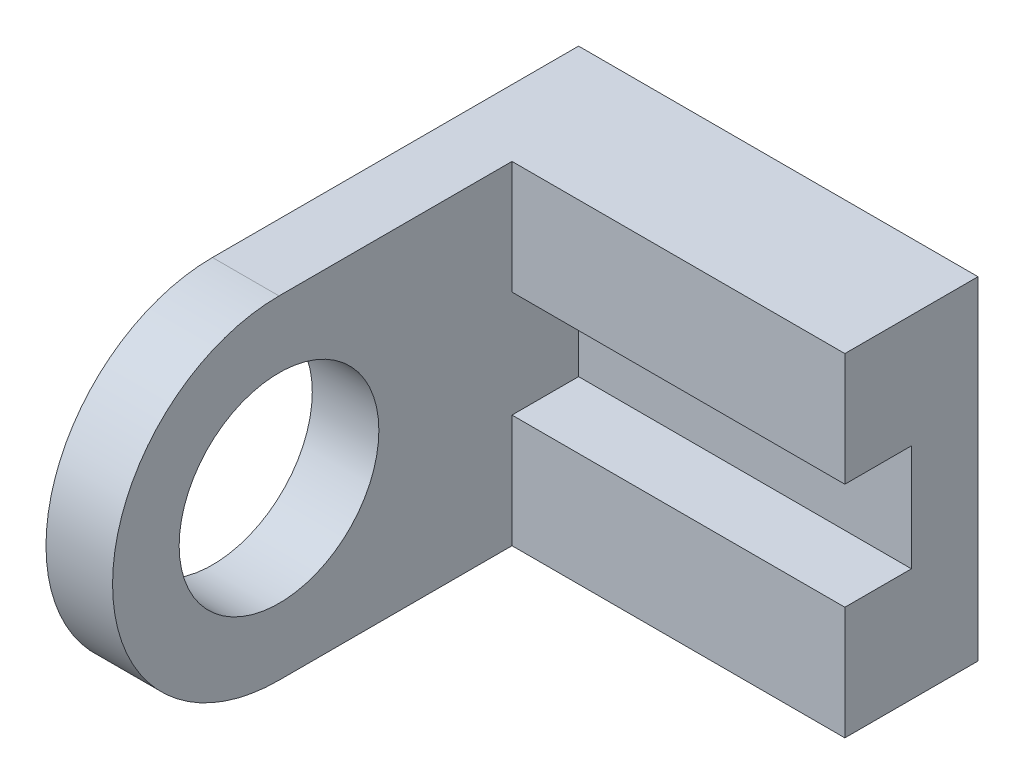
ISO-10303-21;
HEADER;
FILE_DESCRIPTION(('STEP AP214'),'2;1');
FILE_NAME('part.step','',(''),(''),'','','');
FILE_SCHEMA(('AUTOMOTIVE_DESIGN { 1 0 10303 214 1 1 1 1 }'));
ENDSEC;
DATA;
#1=APPLICATION_CONTEXT('core data for automotive mechanical design processes');
#2=APPLICATION_PROTOCOL_DEFINITION('international standard','automotive_design',2000,#1);
#3=PRODUCT_CONTEXT('',#1,'mechanical');
#4=PRODUCT('Part','Part','',(#3));
#5=PRODUCT_RELATED_PRODUCT_CATEGORY('part','',(#4));
#6=PRODUCT_DEFINITION_FORMATION('','',#4);
#7=PRODUCT_DEFINITION_CONTEXT('part definition',#1,'design');
#8=PRODUCT_DEFINITION('design','',#6,#7);
#9=PRODUCT_DEFINITION_SHAPE('','',#8);
#10=(LENGTH_UNIT() NAMED_UNIT(*) SI_UNIT(.MILLI.,.METRE.));
#11=(NAMED_UNIT(*) PLANE_ANGLE_UNIT() SI_UNIT($,.RADIAN.));
#12=(NAMED_UNIT(*) SI_UNIT($,.STERADIAN.) SOLID_ANGLE_UNIT());
#13=UNCERTAINTY_MEASURE_WITH_UNIT(LENGTH_MEASURE(1.E-05),#10,'distance_accuracy_value','');
#14=(GEOMETRIC_REPRESENTATION_CONTEXT(3) GLOBAL_UNCERTAINTY_ASSIGNED_CONTEXT((#13)) GLOBAL_UNIT_ASSIGNED_CONTEXT((#10,
#11,#12)) REPRESENTATION_CONTEXT('',''));
#15=CARTESIAN_POINT('',(0.,0.,0.));
#16=DIRECTION('',(0.,0.,1.));
#17=DIRECTION('',(1.,0.,0.));
#18=AXIS2_PLACEMENT_3D('',#15,#16,#17);
#19=CARTESIAN_POINT('',(0.,0.,10.));
#20=DIRECTION('',(0.,0.,1.));
#21=DIRECTION('',(1.,0.,0.));
#22=AXIS2_PLACEMENT_3D('',#19,#20,#21);
#23=PLANE('',#22);
#24=DIRECTION('',(1.,0.,0.));
#25=VECTOR('',#24,1.);
#26=CARTESIAN_POINT('',(0.,33.,10.));
#27=LINE('',#26,#25);
#28=CARTESIAN_POINT('',(10.,33.,10.));
#29=VERTEX_POINT('',#28);
#30=CARTESIAN_POINT('',(60.,33.,10.));
#31=VERTEX_POINT('',#30);
#32=EDGE_CURVE('E178',#29,#31,#27,.T.);
#33=ORIENTED_EDGE('',*,*,#32,.F.);
#34=DIRECTION('',(0.,-1.,0.));
#35=VECTOR('',#34,1.);
#36=CARTESIAN_POINT('',(10.,50.,10.));
#37=LINE('',#36,#35);
#38=CARTESIAN_POINT('',(10.,17.,10.));
#39=VERTEX_POINT('',#38);
#40=EDGE_CURVE('E131',#29,#39,#37,.T.);
#41=ORIENTED_EDGE('',*,*,#40,.T.);
#42=DIRECTION('',(1.,0.,0.));
#43=VECTOR('',#42,1.);
#44=CARTESIAN_POINT('',(0.,17.,10.));
#45=LINE('',#44,#43);
#46=CARTESIAN_POINT('',(60.,17.,10.));
#47=VERTEX_POINT('',#46);
#48=EDGE_CURVE('E167',#39,#47,#45,.T.);
#49=ORIENTED_EDGE('',*,*,#48,.T.);
#50=DIRECTION('',(0.,1.,0.));
#51=VECTOR('',#50,1.);
#52=CARTESIAN_POINT('',(60.,0.,10.));
#53=LINE('',#52,#51);
#54=EDGE_CURVE('E184',#47,#31,#53,.T.);
#55=ORIENTED_EDGE('',*,*,#54,.T.);
#56=EDGE_LOOP('',(#33,#41,#49,#55));
#57=FACE_BOUND('',#56,.T.);
#58=ADVANCED_FACE('F44',(#57),#23,.T.);
#59=CARTESIAN_POINT('',(0.,50.,10.));
#60=DIRECTION('',(1.,0.,0.));
#61=DIRECTION('',(0.,0.,-1.));
#62=AXIS2_PLACEMENT_3D('',#59,#60,#61);
#63=PLANE('',#62);
#64=CARTESIAN_POINT('',(0.,25.,55.));
#65=DIRECTION('',(1.,0.,0.));
#66=DIRECTION('',(0.,0.,-1.));
#67=AXIS2_PLACEMENT_3D('',#64,#65,#66);
#68=CIRCLE('',#67,15.);
#69=CARTESIAN_POINT('',(0.,25.,40.));
#70=VERTEX_POINT('',#69);
#71=EDGE_CURVE('E153',#70,#70,#68,.T.);
#72=ORIENTED_EDGE('',*,*,#71,.T.);
#73=EDGE_LOOP('',(#72));
#74=FACE_BOUND('',#73,.T.);
#75=DIRECTION('',(0.,0.,-1.));
#76=VECTOR('',#75,1.);
#77=CARTESIAN_POINT('',(0.,0.,10.));
#78=LINE('',#77,#76);
#79=CARTESIAN_POINT('',(0.,0.,55.));
#80=VERTEX_POINT('',#79);
#81=CARTESIAN_POINT('',(0.,0.,0.));
#82=VERTEX_POINT('',#81);
#83=EDGE_CURVE('E52',#80,#82,#78,.T.);
#84=ORIENTED_EDGE('',*,*,#83,.F.);
#85=CARTESIAN_POINT('',(0.,25.,55.));
#86=DIRECTION('',(-1.,0.,0.));
#87=DIRECTION('',(0.,0.,1.));
#88=AXIS2_PLACEMENT_3D('',#85,#86,#87);
#89=CIRCLE('',#88,25.);
#90=CARTESIAN_POINT('',(0.,50.,55.));
#91=VERTEX_POINT('',#90);
#92=EDGE_CURVE('E143',#80,#91,#89,.T.);
#93=ORIENTED_EDGE('',*,*,#92,.T.);
#94=DIRECTION('',(0.,0.,-1.));
#95=VECTOR('',#94,1.);
#96=CARTESIAN_POINT('',(0.,50.,10.));
#97=LINE('',#96,#95);
#98=CARTESIAN_POINT('',(0.,50.,0.));
#99=VERTEX_POINT('',#98);
#100=EDGE_CURVE('E58',#91,#99,#97,.T.);
#101=ORIENTED_EDGE('',*,*,#100,.T.);
#102=DIRECTION('',(0.,-1.,0.));
#103=VECTOR('',#102,1.);
#104=CARTESIAN_POINT('',(0.,50.,0.));
#105=LINE('',#104,#103);
#106=EDGE_CURVE('E179',#99,#82,#105,.T.);
#107=ORIENTED_EDGE('',*,*,#106,.T.);
#108=EDGE_LOOP('',(#84,#93,#101,#107));
#109=FACE_BOUND('',#108,.T.);
#110=ADVANCED_FACE('F50',(#74,#109),#63,.F.);
#111=CARTESIAN_POINT('',(0.,0.,10.));
#112=DIRECTION('',(0.,1.,0.));
#113=DIRECTION('',(0.,0.,1.));
#114=AXIS2_PLACEMENT_3D('',#111,#112,#113);
#115=PLANE('',#114);
#116=DIRECTION('',(1.,0.,0.));
#117=VECTOR('',#116,1.);
#118=CARTESIAN_POINT('',(0.,0.,20.));
#119=LINE('',#118,#117);
#120=CARTESIAN_POINT('',(10.,0.,20.));
#121=VERTEX_POINT('',#120);
#122=CARTESIAN_POINT('',(60.,0.,20.));
#123=VERTEX_POINT('',#122);
#124=EDGE_CURVE('E128',#121,#123,#119,.T.);
#125=ORIENTED_EDGE('',*,*,#124,.F.);
#126=DIRECTION('',(0.,0.,1.));
#127=VECTOR('',#126,1.);
#128=CARTESIAN_POINT('',(10.,0.,10.));
#129=LINE('',#128,#127);
#130=CARTESIAN_POINT('',(10.,0.,55.));
#131=VERTEX_POINT('',#130);
#132=EDGE_CURVE('E122',#121,#131,#129,.T.);
#133=ORIENTED_EDGE('',*,*,#132,.T.);
#134=DIRECTION('',(-1.,0.,0.));
#135=VECTOR('',#134,1.);
#136=CARTESIAN_POINT('',(10.,0.,55.));
#137=LINE('',#136,#135);
#138=EDGE_CURVE('E130',#131,#80,#137,.T.);
#139=ORIENTED_EDGE('',*,*,#138,.T.);
#140=ORIENTED_EDGE('',*,*,#83,.T.);
#141=DIRECTION('',(1.,0.,0.));
#142=VECTOR('',#141,1.);
#143=CARTESIAN_POINT('',(0.,0.,0.));
#144=LINE('',#143,#142);
#145=CARTESIAN_POINT('',(60.,0.,0.));
#146=VERTEX_POINT('',#145);
#147=EDGE_CURVE('E189',#82,#146,#144,.T.);
#148=ORIENTED_EDGE('',*,*,#147,.T.);
#149=DIRECTION('',(0.,0.,-1.));
#150=VECTOR('',#149,1.);
#151=CARTESIAN_POINT('',(60.,0.,10.));
#152=LINE('',#151,#150);
#153=EDGE_CURVE('E198',#123,#146,#152,.T.);
#154=ORIENTED_EDGE('',*,*,#153,.F.);
#155=EDGE_LOOP('',(#125,#133,#139,#140,#148,#154));
#156=FACE_BOUND('',#155,.T.);
#157=ADVANCED_FACE('F127',(#156),#115,.F.);
#158=CARTESIAN_POINT('',(60.,0.,10.));
#159=DIRECTION('',(-1.,0.,0.));
#160=DIRECTION('',(0.,0.,1.));
#161=AXIS2_PLACEMENT_3D('',#158,#159,#160);
#162=PLANE('',#161);
#163=DIRECTION('',(0.,1.,0.));
#164=VECTOR('',#163,1.);
#165=CARTESIAN_POINT('',(60.,0.,0.));
#166=LINE('',#165,#164);
#167=CARTESIAN_POINT('',(60.,50.,0.));
#168=VERTEX_POINT('',#167);
#169=EDGE_CURVE('E68',#146,#168,#166,.T.);
#170=ORIENTED_EDGE('',*,*,#169,.T.);
#171=DIRECTION('',(0.,0.,-1.));
#172=VECTOR('',#171,1.);
#173=CARTESIAN_POINT('',(60.,50.,10.));
#174=LINE('',#173,#172);
#175=CARTESIAN_POINT('',(60.,50.,20.));
#176=VERTEX_POINT('',#175);
#177=EDGE_CURVE('E192',#176,#168,#174,.T.);
#178=ORIENTED_EDGE('',*,*,#177,.F.);
#179=DIRECTION('',(0.,-1.,0.));
#180=VECTOR('',#179,1.);
#181=CARTESIAN_POINT('',(60.,50.,20.));
#182=LINE('',#181,#180);
#183=CARTESIAN_POINT('',(60.,33.,20.));
#184=VERTEX_POINT('',#183);
#185=EDGE_CURVE('E169',#176,#184,#182,.T.);
#186=ORIENTED_EDGE('',*,*,#185,.T.);
#187=DIRECTION('',(0.,0.,-1.));
#188=VECTOR('',#187,1.);
#189=CARTESIAN_POINT('',(60.,33.,20.));
#190=LINE('',#189,#188);
#191=EDGE_CURVE('E174',#184,#31,#190,.T.);
#192=ORIENTED_EDGE('',*,*,#191,.T.);
#193=ORIENTED_EDGE('',*,*,#54,.F.);
#194=DIRECTION('',(0.,0.,1.));
#195=VECTOR('',#194,1.);
#196=CARTESIAN_POINT('',(60.,17.,20.));
#197=LINE('',#196,#195);
#198=CARTESIAN_POINT('',(60.,17.,20.));
#199=VERTEX_POINT('',#198);
#200=EDGE_CURVE('E159',#47,#199,#197,.T.);
#201=ORIENTED_EDGE('',*,*,#200,.T.);
#202=DIRECTION('',(0.,-1.,0.));
#203=VECTOR('',#202,1.);
#204=CARTESIAN_POINT('',(60.,0.,20.));
#205=LINE('',#204,#203);
#206=EDGE_CURVE('E162',#199,#123,#205,.T.);
#207=ORIENTED_EDGE('',*,*,#206,.T.);
#208=ORIENTED_EDGE('',*,*,#153,.T.);
#209=EDGE_LOOP('',(#170,#178,#186,#192,#193,#201,#207,#208));
#210=FACE_BOUND('',#209,.T.);
#211=ADVANCED_FACE('F208',(#210),#162,.F.);
#212=CARTESIAN_POINT('',(60.,50.,10.));
#213=DIRECTION('',(0.,-1.,0.));
#214=DIRECTION('',(0.,0.,-1.));
#215=AXIS2_PLACEMENT_3D('',#212,#213,#214);
#216=PLANE('',#215);
#217=ORIENTED_EDGE('',*,*,#100,.F.);
#218=DIRECTION('',(-1.,0.,0.));
#219=VECTOR('',#218,1.);
#220=CARTESIAN_POINT('',(10.,50.,55.));
#221=LINE('',#220,#219);
#222=CARTESIAN_POINT('',(10.,50.,55.));
#223=VERTEX_POINT('',#222);
#224=EDGE_CURVE('E142',#223,#91,#221,.T.);
#225=ORIENTED_EDGE('',*,*,#224,.F.);
#226=DIRECTION('',(0.,0.,-1.));
#227=VECTOR('',#226,1.);
#228=CARTESIAN_POINT('',(10.,50.,20.));
#229=LINE('',#228,#227);
#230=CARTESIAN_POINT('',(10.,50.,20.));
#231=VERTEX_POINT('',#230);
#232=EDGE_CURVE('E141',#223,#231,#229,.T.);
#233=ORIENTED_EDGE('',*,*,#232,.T.);
#234=DIRECTION('',(1.,0.,0.));
#235=VECTOR('',#234,1.);
#236=CARTESIAN_POINT('',(0.,50.,20.));
#237=LINE('',#236,#235);
#238=EDGE_CURVE('E180',#231,#176,#237,.T.);
#239=ORIENTED_EDGE('',*,*,#238,.T.);
#240=ORIENTED_EDGE('',*,*,#177,.T.);
#241=DIRECTION('',(-1.,0.,0.));
#242=VECTOR('',#241,1.);
#243=CARTESIAN_POINT('',(60.,50.,0.));
#244=LINE('',#243,#242);
#245=EDGE_CURVE('E190',#168,#99,#244,.T.);
#246=ORIENTED_EDGE('',*,*,#245,.T.);
#247=EDGE_LOOP('',(#217,#225,#233,#239,#240,#246));
#248=FACE_BOUND('',#247,.T.);
#249=ADVANCED_FACE('F239',(#248),#216,.F.);
#250=CARTESIAN_POINT('',(0.,0.,0.));
#251=DIRECTION('',(0.,0.,1.));
#252=DIRECTION('',(1.,0.,0.));
#253=AXIS2_PLACEMENT_3D('',#250,#251,#252);
#254=PLANE('',#253);
#255=ORIENTED_EDGE('',*,*,#106,.F.);
#256=ORIENTED_EDGE('',*,*,#245,.F.);
#257=ORIENTED_EDGE('',*,*,#169,.F.);
#258=ORIENTED_EDGE('',*,*,#147,.F.);
#259=EDGE_LOOP('',(#255,#256,#257,#258));
#260=FACE_BOUND('',#259,.T.);
#261=ADVANCED_FACE('F199',(#260),#254,.F.);
#262=CARTESIAN_POINT('',(0.,33.,20.));
#263=DIRECTION('',(0.,-1.,0.));
#264=DIRECTION('',(0.,0.,-1.));
#265=AXIS2_PLACEMENT_3D('',#262,#263,#264);
#266=PLANE('',#265);
#267=DIRECTION('',(0.,0.,1.));
#268=VECTOR('',#267,1.);
#269=CARTESIAN_POINT('',(10.,33.,20.));
#270=LINE('',#269,#268);
#271=CARTESIAN_POINT('',(10.,33.,20.));
#272=VERTEX_POINT('',#271);
#273=EDGE_CURVE('E158',#29,#272,#270,.T.);
#274=ORIENTED_EDGE('',*,*,#273,.F.);
#275=ORIENTED_EDGE('',*,*,#32,.T.);
#276=ORIENTED_EDGE('',*,*,#191,.F.);
#277=DIRECTION('',(1.,0.,0.));
#278=VECTOR('',#277,1.);
#279=CARTESIAN_POINT('',(0.,33.,20.));
#280=LINE('',#279,#278);
#281=EDGE_CURVE('E182',#272,#184,#280,.T.);
#282=ORIENTED_EDGE('',*,*,#281,.F.);
#283=EDGE_LOOP('',(#274,#275,#276,#282));
#284=FACE_BOUND('',#283,.T.);
#285=ADVANCED_FACE('F233',(#284),#266,.T.);
#286=CARTESIAN_POINT('',(0.,50.,20.));
#287=DIRECTION('',(0.,0.,1.));
#288=DIRECTION('',(1.,0.,0.));
#289=AXIS2_PLACEMENT_3D('',#286,#287,#288);
#290=PLANE('',#289);
#291=DIRECTION('',(0.,1.,0.));
#292=VECTOR('',#291,1.);
#293=CARTESIAN_POINT('',(10.,50.,20.));
#294=LINE('',#293,#292);
#295=EDGE_CURVE('E152',#272,#231,#294,.T.);
#296=ORIENTED_EDGE('',*,*,#295,.F.);
#297=ORIENTED_EDGE('',*,*,#281,.T.);
#298=ORIENTED_EDGE('',*,*,#185,.F.);
#299=ORIENTED_EDGE('',*,*,#238,.F.);
#300=EDGE_LOOP('',(#296,#297,#298,#299));
#301=FACE_BOUND('',#300,.T.);
#302=ADVANCED_FACE('F240',(#301),#290,.T.);
#303=CARTESIAN_POINT('',(0.,0.,20.));
#304=DIRECTION('',(0.,0.,1.));
#305=DIRECTION('',(1.,0.,0.));
#306=AXIS2_PLACEMENT_3D('',#303,#304,#305);
#307=PLANE('',#306);
#308=CARTESIAN_POINT('',(10.,17.,20.));
#309=VERTEX_POINT('',#308);
#310=EDGE_CURVE('E156',#121,#309,#294,.T.);
#311=ORIENTED_EDGE('',*,*,#310,.F.);
#312=ORIENTED_EDGE('',*,*,#124,.T.);
#313=ORIENTED_EDGE('',*,*,#206,.F.);
#314=DIRECTION('',(1.,0.,0.));
#315=VECTOR('',#314,1.);
#316=CARTESIAN_POINT('',(0.,17.,20.));
#317=LINE('',#316,#315);
#318=EDGE_CURVE('E166',#309,#199,#317,.T.);
#319=ORIENTED_EDGE('',*,*,#318,.F.);
#320=EDGE_LOOP('',(#311,#312,#313,#319));
#321=FACE_BOUND('',#320,.T.);
#322=ADVANCED_FACE('F253',(#321),#307,.T.);
#323=CARTESIAN_POINT('',(0.,17.,20.));
#324=DIRECTION('',(0.,1.,0.));
#325=DIRECTION('',(0.,0.,1.));
#326=AXIS2_PLACEMENT_3D('',#323,#324,#325);
#327=PLANE('',#326);
#328=DIRECTION('',(0.,0.,-1.));
#329=VECTOR('',#328,1.);
#330=CARTESIAN_POINT('',(10.,17.,20.));
#331=LINE('',#330,#329);
#332=EDGE_CURVE('E11',#309,#39,#331,.T.);
#333=ORIENTED_EDGE('',*,*,#332,.F.);
#334=ORIENTED_EDGE('',*,*,#318,.T.);
#335=ORIENTED_EDGE('',*,*,#200,.F.);
#336=ORIENTED_EDGE('',*,*,#48,.F.);
#337=EDGE_LOOP('',(#333,#334,#335,#336));
#338=FACE_BOUND('',#337,.T.);
#339=ADVANCED_FACE('F227',(#338),#327,.T.);
#340=CARTESIAN_POINT('',(10.,25.,55.));
#341=DIRECTION('',(-1.,0.,0.));
#342=DIRECTION('',(0.,0.,1.));
#343=AXIS2_PLACEMENT_3D('',#340,#341,#342);
#344=CYLINDRICAL_SURFACE('',#343,25.);
#345=ORIENTED_EDGE('',*,*,#92,.F.);
#346=ORIENTED_EDGE('',*,*,#138,.F.);
#347=CARTESIAN_POINT('',(10.,25.,55.));
#348=DIRECTION('',(-1.,0.,0.));
#349=DIRECTION('',(0.,0.,1.));
#350=AXIS2_PLACEMENT_3D('',#347,#348,#349);
#351=CIRCLE('',#350,25.);
#352=EDGE_CURVE('E134',#131,#223,#351,.T.);
#353=ORIENTED_EDGE('',*,*,#352,.T.);
#354=ORIENTED_EDGE('',*,*,#224,.T.);
#355=EDGE_LOOP('',(#345,#346,#353,#354));
#356=FACE_BOUND('',#355,.T.);
#357=ADVANCED_FACE('F137',(#356),#344,.T.);
#358=CARTESIAN_POINT('',(10.,25.,55.));
#359=DIRECTION('',(-1.,0.,0.));
#360=DIRECTION('',(0.,0.,1.));
#361=AXIS2_PLACEMENT_3D('',#358,#359,#360);
#362=PLANE('',#361);
#363=CARTESIAN_POINT('',(10.,25.,55.));
#364=DIRECTION('',(1.,0.,0.));
#365=DIRECTION('',(0.,0.,-1.));
#366=AXIS2_PLACEMENT_3D('',#363,#364,#365);
#367=CIRCLE('',#366,15.);
#368=CARTESIAN_POINT('',(10.,25.,40.));
#369=VERTEX_POINT('',#368);
#370=EDGE_CURVE('E212',#369,#369,#367,.T.);
#371=ORIENTED_EDGE('',*,*,#370,.F.);
#372=EDGE_LOOP('',(#371));
#373=FACE_BOUND('',#372,.T.);
#374=ORIENTED_EDGE('',*,*,#273,.T.);
#375=ORIENTED_EDGE('',*,*,#295,.T.);
#376=ORIENTED_EDGE('',*,*,#232,.F.);
#377=ORIENTED_EDGE('',*,*,#352,.F.);
#378=ORIENTED_EDGE('',*,*,#132,.F.);
#379=ORIENTED_EDGE('',*,*,#310,.T.);
#380=ORIENTED_EDGE('',*,*,#332,.T.);
#381=ORIENTED_EDGE('',*,*,#40,.F.);
#382=EDGE_LOOP('',(#374,#375,#376,#377,#378,#379,#380,#381));
#383=FACE_BOUND('',#382,.T.);
#384=ADVANCED_FACE('F148',(#373,#383),#362,.F.);
#385=CARTESIAN_POINT('',(0.,25.,55.));
#386=DIRECTION('',(1.,0.,0.));
#387=DIRECTION('',(0.,0.,-1.));
#388=AXIS2_PLACEMENT_3D('',#385,#386,#387);
#389=CYLINDRICAL_SURFACE('',#388,15.);
#390=ORIENTED_EDGE('',*,*,#71,.F.);
#391=EDGE_LOOP('',(#390));
#392=FACE_BOUND('',#391,.T.);
#393=ORIENTED_EDGE('',*,*,#370,.T.);
#394=EDGE_LOOP('',(#393));
#395=FACE_BOUND('',#394,.T.);
#396=ADVANCED_FACE('F263',(#392,#395),#389,.F.);
#397=CLOSED_SHELL('',(#58,#110,#157,#211,#249,#261,#285,#302,#322,#339,#357,#384,#396));
#398=MANIFOLD_SOLID_BREP('B2',#397);
#399=ADVANCED_BREP_SHAPE_REPRESENTATION('',(#18,#398),#14);
#400=SHAPE_DEFINITION_REPRESENTATION(#9,#399);
ENDSEC;
END-ISO-10303-21;
